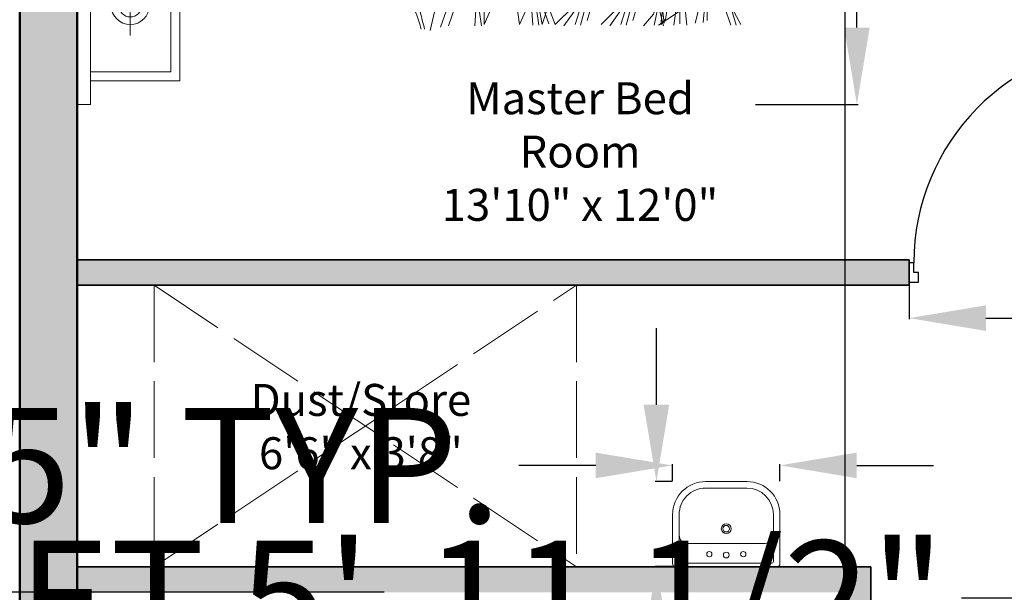
# Model space of a CAD drawing. Units: inches. Extents: x 2796 to 3603, y 978 to 1787.
# Tile 9 of 15: x 3070 to 3224, y 1456 to 1545. Entities that reach past the tile are written whole.
import ezdxf

# ---------------------------------------------------------------- set-up
doc = ezdxf.new("R2010")
doc.units = ezdxf.units.IN
doc.linetypes.add('ACAD_ISO02W100', pattern=[15, 12, -3])
for name, color, linetype, lineweight in [('A-ANNO-DIMS', 7, 'Continuous', 18), ('A-AREA-IDEN', 7, 'Continuous', 18), ('A-DOOR', 6, 'Continuous', 25), ('A-FLOR-FIXT', 8, 'Continuous', 18), ('A-FLOR-OVHD', 7, 'ACAD_ISO02W100', 18), ('A-WALL-EXTR-PATT', 1, 'Continuous', 13), ('A-WALL-INTR-PATT', 5, 'Continuous', 13), ('Furniture', 2, 'Continuous', 18), ('Inner Wall', 5, 'Continuous', 35), ('Outer Wall', 1, 'Continuous', 50)]:
    doc.layers.add(name, color=color, linetype=linetype, lineweight=lineweight)
doc.styles.get("Standard").update_dxf_attribs({"font": 'arial.ttf'})
doc.dimstyles.get("Standard").update_dxf_attribs({"dimtxt": 18, "dimasz": 12, "dimexe": 0.18, "dimexo": 0.0625, "dimgap": 0.09, "dimtad": 0, "dimtih": 1, "dimtoh": 1, "dimdec": 0, "dimzin": 0, "dimdsep": 46, "dimlunit": 3, "dimtxsty": 'Standard', "dimcen": 0.09, "dimadec": 0, "dimazin": 0, "dimtfac": 1, "dimtdec": 0, "dimtofl": 0, "dimtmove": 0, "dimatfit": 3, "dimfxl": 1, "dimtolj": 1, "dimtzin": 0, "dimarcsym": 0})

# ---------------------------------------------------------------- blocks, each defined once
blk = doc.blocks.new('A$C57EA129C')
for p, q in [((0, 0.4428), (0, 0.1782)), ((0.016, 0.4589), (0.5631, 0.4589)), ((0.0356, 0.4321), (0.0356, 0.2896)), ((0.0445, 0.441), (0.5346, 0.441)), ((0.5435, 0.4321), (0.5435, 0.2896)), ((0.5791, 0.4428), (0.5791, 0.1782)), ((0.0802, 0.3341), (0.499, 0.3341)), ((0.0356, 0.2896), (0.0356, 0.1782)), ((0.5435, 0.2896), (0.5435, 0.1782)), ((0.1782, 0.0356), (0.4009, 0.0356)), ((0.1782, 0), (0.4009, 0))]:
    blk.add_line(p, q)
for centre, radius in [((0.1982, 0.392), 0.0143), ((0.2896, 0.3965), 0.0156), ((0.3809, 0.392), 0.0143), ((0.2896, 0.2545), 0.0267), ((0.2896, 0.2545), 0.0178)]:
    blk.add_circle(centre, radius)
for centre, radius, start, end in [((0.016, 0.4428), 0.016, 90, 180), ((0.0445, 0.4321), 0.00891, 90, 180), ((0.5346, 0.4321), 0.00891, 0, 90), ((0.5631, 0.4428), 0.016, 0, 90), ((0.0802, 0.2896), 0.0445, 90, 180), ((0.499, 0.2896), 0.0445, 0, 90), ((0.1782, 0.1782), 0.1782, 180, 270), ((0.1782, 0.1782), 0.1426, 180, 270), ((0.4009, 0.1782), 0.1782, 270, 0), ((0.4009, 0.1782), 0.1426, 270, 0)]:
    blk.add_arc(centre, radius, start, end)
blk = doc.blocks.new('A$C2B723114')
for p, q in [((0, 2.9047), (2.8274, 2.9047)), ((0, 2.8487), (0, 2.9047)), ((0.4243, 2.8697), (0.4243, 2.4855)), ((2.4742, 2.8697), (2.4742, 2.4855)), ((2.8274, 2.9047), (2.8274, 2.8487)), ((2.8274, 2.8487), (0, 2.8487)), ((0.1012, 2.4649), (0.1012, 2.849)), ((0.1396, 2.5033), (0.1396, 2.849)), ((0.6794, 0.7051), (0.6794, 2.8509)), ((0.7187, 0.7435), (0.7187, 2.8509)), ((2.1776, 2.8509), (2.1776, 0.7454)), ((2.216, 2.8509), (2.216, 0.707)), ((2.6798, 2.5052), (2.6798, 2.8509)), ((2.7182, 2.4668), (2.7182, 2.8509)), ((0.6087, 2.6776), (0.295, 2.6776)), ((2.6586, 2.6776), (2.2821, 2.6776)), ((1.3789, 2.4999), (1.3598, 2.5761)), ((2.0593, 2.4999), (2.0402, 2.5761)), ((0.6766, 2.5033), (0.1396, 2.5033)), ((1.3858, 2.4723), (1.3789, 2.4999)), ((2.0662, 2.4723), (2.0593, 2.4999)), ((2.2188, 2.5052), (2.6798, 2.5052)), ((0.6794, 2.4649), (0.1012, 2.4649)), ((0.7191, 2.47), (2.1778, 2.4719)), ((2.2188, 2.4668), (2.7182, 2.4668)), ((2.1771, 2.3036), (0.718, 2.1685)), ((1.0365, 1.6233), (2.1246, 2.2989)), ((2.2287, 1.6076), (2.2523, 1.5035)), ((0.5047, 1.5819), (0.5353, 1.4945)), ((0.6174, 1.5819), (0.6232, 1.4916)), ((0.6467, 1.5819), (0.6369, 1.5137)), ((0.6571, 1.4945), (0.6571, 1.5765)), ((2.2726, 1.593), (2.3061, 1.5007)), ((2.3067, 1.5881), (2.3373, 1.5007)), ((2.4194, 1.5881), (2.4251, 1.4979)), ((2.4487, 1.5881), (2.4389, 1.5199)), ((2.4591, 1.5007), (2.4591, 1.5828)), ((0.4269, 0.0884), (0.4269, 1.4945)), ((0.4269, 1.4945), (0.6794, 1.4945)), ((2.4685, 1.4964), (2.216, 1.5022)), ((2.4685, 1.4964), (2.4685, 0.0903)), ((0.3172, 1.3923), (0.4213, 1.3687)), ((2.4685, 1.4044), (2.5491, 1.3861)), ((2.4596, 1.3659), (2.552, 1.3324)), ((0.3318, 1.3485), (0.4241, 1.3149)), ((0.3367, 1.3143), (0.4241, 1.2838)), ((2.4645, 1.3318), (2.552, 1.3012)), ((2.4645, 1.2928), (2.5548, 1.2871)), ((2.4645, 1.2635), (2.5328, 1.2733)), ((2.4699, 1.2531), (2.552, 1.2163)), ((2.552, 1.2531), (2.4699, 1.2531)), ((2.5435, 1.2276), (2.4699, 1.2163)), ((0.3367, 1.2016), (0.427, 1.1959)), ((0.3367, 1.1724), (0.405, 1.1821)), ((2.4699, 1.2163), (2.5463, 1.1823)), ((0.4241, 1.162), (0.3421, 1.162)), ((0.3421, 1.162), (0.4241, 1.1252)), ((2.5491, 1.1654), (2.467, 1.1597)), ((2.5463, 1.1455), (2.467, 1.1342)), ((2.5491, 1.1342), (2.4699, 1.1201)), ((2.4699, 1.1201), (2.5491, 1.0946)), ((2.5463, 1.1172), (2.4727, 1.0918)), ((2.5491, 1.0946), (2.4699, 1.0635)), ((2.4699, 1.0635), (2.5491, 0.9842)), ((0.4157, 1.0206), (0.3421, 1.0093)), ((2.4642, 1.0267), (2.552, 0.9644)), ((0.3421, 1.0093), (0.4185, 0.9754)), ((2.4699, 0.9785), (2.552, 0.9531)), ((0.4213, 0.9584), (0.3392, 0.9527)), ((0.4185, 0.9386), (0.3392, 0.9272)), ((2.4642, 0.9389), (2.4869, 0.9276)), ((2.467, 0.9559), (2.552, 0.9333)), ((0.4213, 0.9272), (0.3421, 0.9131)), ((0.3421, 0.9131), (0.4213, 0.8876)), ((0.4213, 0.8876), (0.3421, 0.8565)), ((0.4185, 0.9103), (0.3449, 0.8848)), ((2.4642, 0.8908), (2.5152, 0.8483)), ((2.4869, 0.9276), (2.5265, 0.9163)), ((2.5265, 0.9163), (2.5491, 0.9163)), ((0.3421, 0.8565), (0.4213, 0.7772)), ((2.467, 0.8455), (2.5208, 0.8342)), ((2.5152, 0.8483), (2.5491, 0.837)), ((0.3364, 0.8197), (0.4241, 0.7574)), ((2.4699, 0.8172), (2.4925, 0.7974)), ((2.5491, 0.8087), (2.4699, 0.8172)), ((2.5208, 0.8342), (2.552, 0.8285)), ((2.552, 0.8285), (2.5293, 0.8087)), ((0.3421, 0.7716), (0.4241, 0.7461)), ((2.5491, 0.7606), (2.467, 0.7719)), ((2.4925, 0.7974), (2.535, 0.7889)), ((2.535, 0.7889), (2.552, 0.7861)), ((0.3392, 0.7489), (0.4241, 0.7263)), ((0.359, 0.7206), (0.3987, 0.7093)), ((2.1776, 0.7454), (0.7187, 0.7435)), ((2.4727, 0.7464), (2.467, 0.7408)), ((2.467, 0.7153), (2.5491, 0.7238)), ((2.552, 0.7464), (2.4727, 0.7464)), ((0.3987, 0.7093), (0.4213, 0.7093)), ((2.216, 0.707), (0.6794, 0.7051)), ((0.9938, 0.6115), (1.7555, 0.7064)), ((2.5491, 0.6842), (2.4642, 0.6615)), ((2.552, 0.7096), (2.467, 0.6842)), ((0.3421, 0.6601), (0.4213, 0.5808)), ((2.5491, 0.6672), (2.4755, 0.6587)), ((2.4755, 0.6474), (2.5548, 0.6276)), ((0.3364, 0.6233), (0.4241, 0.561)), ((2.4642, 0.6191), (2.4784, 0.6134)), ((2.467, 0.5993), (2.4869, 0.5964)), ((2.4784, 0.6134), (2.5406, 0.6077)), ((2.4869, 0.5964), (2.552, 0.5964)), ((2.5406, 0.6077), (2.552, 0.6134)), ((0.3392, 0.5525), (0.4241, 0.5299)), ((0.3421, 0.5752), (0.4241, 0.5497)), ((2.467, 0.5313), (2.5491, 0.5596)), ((0.359, 0.5242), (0.3987, 0.5129)), ((2.467, 0.5087), (2.5548, 0.5342)), ((2.5548, 0.5342), (2.4699, 0.4889)), ((0.3364, 0.4785), (0.3874, 0.436)), ((1.4523, 0.5021), (1.1305, 0.4537)), ((0.3392, 0.4332), (0.393, 0.4219)), ((0.3874, 0.436), (0.4213, 0.4247)), ((1.1305, 0.4537), (0.9938, 0.448)), ((0.4213, 0.415), (0.3364, 0.3923)), ((0.4241, 0.2868), (0.3392, 0.415)), ((0.3421, 0.4049), (0.3647, 0.3851)), ((0.4213, 0.3964), (0.3421, 0.4049)), ((0.4213, 0.398), (0.3477, 0.3895)), ((0.3647, 0.3851), (0.4072, 0.3766)), ((0.393, 0.4219), (0.4241, 0.4162)), ((0.4241, 0.4162), (0.4015, 0.3964)), ((2.467, 0.4133), (2.552, 0.4019)), ((2.467, 0.2879), (2.552, 0.4076)), ((0.4213, 0.3377), (0.3392, 0.3491)), ((0.4072, 0.3766), (0.4241, 0.3738)), ((0.3392, 0.2925), (0.4213, 0.3009)), ((0.4241, 0.3236), (0.3449, 0.3236)), ((2.4642, 0.3049), (2.5491, 0.2851)), ((2.467, 0.319), (2.5548, 0.3134)), ((0.3477, 0.2571), (0.427, 0.2373)), ((2.501, 0.2491), (2.5491, 0.2547)), ((0.3506, 0.2231), (0.4128, 0.2175)), ((0.4128, 0.2175), (0.4241, 0.2231)), ((2.467, 0.2179), (2.5605, 0.1981)), ((2.4699, 0.2491), (2.501, 0.2491)), ((0.359, 0.2061), (0.4241, 0.2061)), ((2.467, 0.1981), (2.5491, 0.1613)), ((2.467, 0.184), (2.4982, 0.1755)), ((2.4982, 0.1755), (2.5463, 0.1359)), ((0.3392, 0.1042), (0.4213, 0.1325)), ((2.4699, 0.1302), (2.535, 0.1104)), ((0.3392, 0.0815), (0.427, 0.107)), ((0.427, 0.107), (0.3421, 0.0617)), ((2.4685, 0.0903), (0.4269, 0.0884)), ((0.5106, 0.094), (0.5106, 0.0657)), ((0.5417, 0.094), (0.5474, 0.0572)), ((0.587, 0.0884), (0.604, 0.0346)), ((0.6512, 0.0884), (0.6682, 0.0346)), ((0.713, 0.094), (0.713, 0.0657)), ((0.7334, 0.0943), (0.7503, 0.0434)), ((0.7786, 0.0915), (0.7786, 0.0632)), ((0.8739, 0.0884), (0.8908, 0.0346)), ((0.956, 0.0943), (0.973, 0.0434)), ((1.0013, 0.0915), (1.0013, 0.0632)), ((1.072, 0.0884), (1.089, 0.0346)), ((1.1338, 0.094), (1.1338, 0.0657)), ((1.1542, 0.0943), (1.1712, 0.0434)), ((1.1995, 0.0915), (1.1995, 0.0632)), ((1.4088, 0.094), (1.4088, 0.0657)), ((1.44, 0.094), (1.4456, 0.0572)), ((1.4853, 0.0884), (1.5023, 0.0346)), ((1.5674, 0.0962), (1.5844, 0.0453)), ((1.6127, 0.0934), (1.6127, 0.0651)), ((1.6297, 0.0849), (1.624, 0.0028)), ((1.6721, 0.0877), (1.6693, 0.0623)), ((1.7344, 0.0934), (1.7344, 0.0651)), ((1.7655, 0.0934), (1.7712, 0.0566)), ((1.8108, 0.0877), (1.8278, 0.034)), ((1.8568, 0.0962), (1.8738, 0.0453)), ((1.9342, 0.0962), (1.9512, 0.0453)), ((1.9795, 0.0934), (1.9795, 0.0651)), ((1.9965, 0.0849), (1.9908, 0.0028)), ((2.039, 0.0877), (2.0361, 0.0623)), ((2.1012, 0.0934), (2.1012, 0.0651)), ((2.1324, 0.0934), (2.138, 0.0566)), ((2.1777, 0.0877), (2.1946, 0.034)), ((2.2236, 0.0962), (2.2406, 0.0453)), ((2.2689, 0.0934), (2.2689, 0.0651)), ((2.2859, 0.0849), (2.2802, 0.0028)), ((2.3284, 0.0877), (2.3255, 0.0623)), ((2.3906, 0.0934), (2.3906, 0.0651)), ((2.4218, 0.0934), (2.4274, 0.0566)), ((2.4642, 0.0991), (2.5378, 0.0877)), ((2.467, 0.0877), (2.484, 0.034)), ((2.535, 0.1104), (2.5491, 0.0991)), ((2.5378, 0.0877), (2.5463, 0.0821)), ((0.5106, 0.0657), (0.5077, 0.0063)), ((0.5474, 0.0572), (0.57, 0.0006)), ((0.713, 0.0657), (0.7101, 0.0063)), ((0.7503, 0.0434), (0.773, 0.0037)), ((0.7786, 0.0632), (0.7843, 0.0066)), ((0.973, 0.0434), (0.9957, 0.0037)), ((1.0013, 0.0632), (1.007, 0.0066)), ((1.1338, 0.0657), (1.131, 0.0063)), ((1.1712, 0.0434), (1.1939, 0.0037)), ((1.1995, 0.0632), (1.2052, 0.0066)), ((1.4088, 0.0657), (1.406, 0.0063)), ((1.4456, 0.0572), (1.4683, 0.0006)), ((1.5844, 0.0453), (1.607, 0.0057)), ((1.6127, 0.0651), (1.6184, 0.0085)), ((1.6693, 0.0623), (1.6608, 0.0028)), ((1.7344, 0.0651), (1.7316, 0.0057)), ((1.7712, 0.0566), (1.7938, 0)), ((1.8738, 0.0453), (1.8964, 0.0057)), ((1.9512, 0.0453), (1.9739, 0.0057)), ((1.9795, 0.0651), (1.9852, 0.0085)), ((2.0361, 0.0623), (2.0276, 0.0028)), ((2.1012, 0.0651), (2.0984, 0.0057)), ((2.138, 0.0566), (2.1607, 0)), ((2.2406, 0.0453), (2.2632, 0.0057)), ((2.2689, 0.0651), (2.2746, 0.0085)), ((2.3255, 0.0623), (2.317, 0.0028)), ((2.3906, 0.0651), (2.3878, 0.0057)), ((2.4274, 0.0566), (2.4501, 0)), ((0.604, 0.0346), (0.621, 0.0063)), ((0.6682, 0.0346), (0.6851, 0.0063)), ((0.8908, 0.0346), (0.9078, 0.0063)), ((1.089, 0.0346), (1.106, 0.0063)), ((1.5023, 0.0346), (1.5192, 0.0082)), ((1.8278, 0.034), (1.8448, 0.0057)), ((2.1946, 0.034), (2.2116, 0.0057)), ((2.484, 0.034), (2.501, 0.0057))]:
    blk.add_line(p, q)
for centre, radius in [((0.4243, 2.6776), 0.0821), ((2.4742, 2.6776), 0.0821), ((0.4243, 2.6776), 0.0493), ((2.4742, 2.6776), 0.0493)]:
    blk.add_circle(centre, radius)
for centre, radius, start, end in [((0.8078, 2.821), 0.00214, 160.436, 281.8931), ((0.8088, 2.8207), 0.00315, 111.7883, 160.436), ((0.8162, 2.8021), 0.0232, 94.3025, 111.7883), ((0.8091, 2.8151), 0.00394, 21.9904, 101.8931), ((0.8409, 2.7949), 0.0302, 158.579, 188.1335), ((1.0356, 2.8227), 0.2268, 188.1335, 192.1095), ((0.7994, 2.8112), 0.0144, 338.579, 21.9904), ((0.8165, 2.7987), 0.0266, 59.3487, 94.3025), ((0.8554, 2.8643), 0.0497, 239.3487, 264.7408), ((0.9202, 3.5684), 0.7568, 264.7408, 268.0921), ((0.8679, 2.7254), 0.0915, 74.0648, 94.2159), ((0.8679, 2.7254), 0.0915, 53.9136, 74.0648), ((0.9409, 4.189), 1.3777, 268.0921, 270.5757), ((0.8679, 2.7254), 0.0915, 36.1766, 53.9136), ((0.86, 2.6097), 0.2158, 62.7604, 69.1397), ((0.9466, 3.6164), 0.8051, 270.5757, 274.8018), ((0.9263, 2.7386), 0.0708, 51.6114, 62.7604), ((0.7461, 2.511), 0.3611, 46.1885, 51.6114), ((1.0364, 2.548), 0.2671, 87.4614, 94.8018), ((1.042, 2.6745), 0.1405, 79.8101, 87.4614), ((1.1532, 3.2931), 0.488, 259.8101, 263.9133), ((1.204, 3.7695), 0.9671, 263.9133, 270), ((1.204, 3.4318), 0.6294, 270, 277.5469), ((1.2573, 3.0292), 0.2233, 277.5469, 285.744), ((1.3941, 2.5438), 0.281, 98.4372, 105.744), ((1.3747, 2.6748), 0.1486, 90, 98.4372), ((1.3713, 2.8186), 0.0315, 274.4002, 333.4195), ((0.923, 2.7382), 0.4535, 0, 6.2324), ((1.3747, 2.74), 0.0833, 78.7276, 90), ((1.3886, 2.8099), 0.0121, 333.4195, 78.7276), ((1.4882, 2.821), 0.00214, 160.436, 281.8931), ((1.4892, 2.8207), 0.00315, 111.7883, 160.436), ((1.4966, 2.8021), 0.0232, 94.3025, 111.7883), ((1.4895, 2.8151), 0.00394, 21.9904, 101.8931), ((1.5213, 2.7949), 0.0302, 158.579, 188.1335), ((1.716, 2.8227), 0.2268, 188.1335, 192.1095), ((1.4798, 2.8112), 0.0144, 338.579, 21.9904), ((1.4969, 2.7987), 0.0266, 59.3487, 94.3025), ((1.5358, 2.8643), 0.0497, 239.3487, 264.7408), ((1.6006, 3.5684), 0.7568, 264.7408, 268.0921), ((1.5483, 2.7254), 0.0915, 74.0648, 94.2159), ((1.5483, 2.7254), 0.0915, 53.9136, 74.0648), ((1.6213, 4.189), 1.3777, 268.0921, 270.5757), ((1.5483, 2.7254), 0.0915, 36.1766, 53.9136), ((1.5404, 2.6097), 0.2158, 62.7604, 69.1397), ((1.627, 3.6164), 0.8051, 270.5757, 274.8018), ((1.6067, 2.7386), 0.0708, 51.6114, 62.7604), ((1.4265, 2.511), 0.3611, 46.1885, 51.6114), ((1.7168, 2.548), 0.2671, 87.4614, 94.8018), ((1.7224, 2.6745), 0.1405, 79.8101, 87.4614), ((1.8336, 3.2931), 0.488, 259.8101, 263.9133), ((1.8844, 3.7695), 0.9671, 263.9133, 270), ((1.8844, 3.4318), 0.6294, 270, 277.5469), ((1.9377, 3.0292), 0.2233, 277.5469, 285.744), ((2.0745, 2.5438), 0.281, 98.4372, 105.744), ((2.0551, 2.6748), 0.1486, 90, 98.4372), ((2.0517, 2.8186), 0.0315, 274.4002, 333.4195), ((1.6034, 2.7382), 0.4535, 0, 6.2324), ((2.0551, 2.74), 0.0833, 78.7276, 90), ((2.069, 2.8099), 0.0121, 333.4195, 78.7276), ((0.635, 2.7368), 0.1829, 7.6809, 12.1095), ((-0.0181, 2.6487), 0.8418, 3.3687, 7.6809), ((0.8679, 2.7254), 0.0915, 18.4397, 36.1766), ((0.8523, 2.6218), 0.2076, 39.0349, 46.1885), ((0.9783, 2.7239), 0.0455, 28.3168, 39.0349), ((0.8558, 2.6579), 0.1846, 23.0028, 28.3168), ((1.3154, 2.7368), 0.1829, 7.6809, 12.1095), ((0.6623, 2.6487), 0.8418, 3.3687, 7.6809), ((1.5483, 2.7254), 0.0915, 18.4397, 36.1766), ((1.5327, 2.6218), 0.2076, 39.0349, 46.1885), ((1.6587, 2.7239), 0.0455, 28.3168, 39.0349), ((1.5362, 2.6579), 0.1846, 23.0028, 28.3168), ((0.5722, 2.8434), 0.8132, 347.8016, 350.3156), ((1.1884, 2.7382), 0.1881, 350.3156, 0), ((1.2526, 2.8434), 0.8132, 347.8016, 350.3156), ((1.8688, 2.7382), 0.1881, 350.3156, 0), ((0.1976, 2.6614), 0.6258, 358.3669, 3.3687), ((1.6528, 2.6098), 0.2924, 167.8016, 171.9949), ((0.878, 2.6614), 0.6258, 358.3669, 3.3687), ((2.3332, 2.6098), 0.2924, 167.8016, 171.9949), ((-0.4351, 2.6794), 1.2587, 356.945, 358.3669), ((1.9648, 2.5659), 0.6074, 171.9949, 177.3351), ((0.2453, 2.6794), 1.2587, 356.945, 358.3669), ((2.6452, 2.5659), 0.6074, 171.9949, 177.3351), ((-11.7321, 3.2823), 12.5718, 356.49514, 356.94504), ((1.4204, 2.5912), 0.0624, 177.3351, 194.0452), ((-11.0517, 3.2823), 12.5718, 356.49514, 356.94504), ((2.1008, 2.5912), 0.0624, 177.3351, 194.0452), ((0.5206, 2.5319), 0.2961, 350.0016, 356.4951), ((1.4917, 3.1364), 0.681, 244.6889, 246.5156), ((1.4917, 3.1364), 0.681, 246.5156, 248.3423), ((1.4917, 3.1364), 0.681, 248.3423, 250.572), ((1.4917, 3.1364), 0.681, 250.572, 252.8018), ((1.201, 2.5319), 0.2961, 350.0016, 356.4951), ((2.1721, 3.1364), 0.681, 244.6889, 246.5156), ((2.1721, 3.1364), 0.681, 246.5156, 248.3423), ((2.1721, 3.1364), 0.681, 248.3423, 250.572), ((2.1721, 3.1364), 0.681, 250.572, 252.8018), ((0.8298, 2.4774), 0.0178, 170.0016, 196.6978), ((0.8139, 2.4726), 0.00122, 196.6978, 277.1204), ((0.8041, 2.5514), 0.0807, 277.1204, 286.2212), ((0.8068, 2.5419), 0.0707, 286.2212, 297.2841), ((0.8584, 2.4419), 0.0418, 102.869, 117.2841), ((0.879, 2.3515), 0.1345, 93.574, 102.869), ((0.9376, 1.4146), 1.0732, 90.2865, 93.574), ((0.9586, -2.7845), 5.2724, 89.0296, 90.2865), ((0.9954, -0.6123), 3.0999, 87.3904, 89.0296), ((1.0854, 1.364), 1.1216, 85.3824, 87.3904), ((1.28, 3.7729), 1.2952, 265.3824, 267.2509), ((1.228, 2.691), 0.2121, 267.2509, 281.5586), ((1.2975, 2.3514), 0.1345, 83.5659, 101.5586), ((1.3002, 2.3754), 0.1104, 72.6136, 83.5659), ((1.3965, 2.6828), 0.2118, 252.6136, 260.5159), ((1.4027, 2.7202), 0.2496, 260.5159, 265.9171), ((1.385, 2.4721), 0.000845, 265.9171, 14.0449), ((1.5102, 2.4774), 0.0178, 170.0016, 196.6978), ((1.4943, 2.4726), 0.00122, 196.6978, 277.1204), ((1.4845, 2.5514), 0.0807, 277.1204, 286.2212), ((1.4872, 2.5419), 0.0707, 286.2212, 297.2841), ((1.5388, 2.4419), 0.0418, 102.869, 117.2841), ((1.5594, 2.3515), 0.1345, 93.574, 102.869), ((1.618, 1.4146), 1.0732, 90.2865, 93.574), ((1.639, -2.7845), 5.2724, 89.0296, 90.2865), ((1.6758, -0.6123), 3.0999, 87.3904, 89.0296), ((1.7658, 1.364), 1.1216, 85.3824, 87.3904), ((1.9604, 3.7729), 1.2952, 265.3824, 267.2509), ((1.9084, 2.691), 0.2121, 267.2509, 281.5586), ((1.9779, 2.3514), 0.1345, 83.5659, 101.5586), ((1.9806, 2.3754), 0.1104, 72.6136, 83.5659), ((2.0769, 2.6828), 0.2118, 252.6136, 260.5159), ((2.0831, 2.7202), 0.2496, 260.5159, 265.9171), ((2.0654, 2.4721), 0.000845, 265.9171, 14.0449)]:
    blk.add_arc(centre, radius, start, end)
blk.add_ellipse((0.4962, 1.9132), major_axis=(0.4887, -0.4605), ratio=0.503305, start_param=0.491272, end_param=1.591113)
for points, knots in [([(0.6768, 1.3104), (0.6615, 1.3339), (0.6315, 1.3797), (0.604, 1.4501), (0.5417, 1.4748), (0.5064, 1.4871), (0.4848, 1.4945)], [0, 0, 0, 0, 110.980521, 216.571322, 273.316778, 363.252298, 363.252298, 363.252298, 363.252298]), ([(2.5548, 1.4853), (2.5314, 1.4757), (2.5031, 1.4641), (2.4737, 1.4555), (2.4685, 1.454)], [0, 0, 0, 0, 98.452083, 119.481049, 119.481049, 119.481049, 119.481049]), ([(0.427, 1.4678), (0.4036, 1.4582), (0.3693, 1.4441), (0.3335, 1.4344), (0.3221, 1.4313)], [0, 0, 0, 0, 98.452083, 144.639601, 144.639601, 144.639601, 144.639601]), ([(0.4241, 1.4423), (0.4031, 1.437), (0.3691, 1.4284), (0.3351, 1.4199), (0.3221, 1.4167)], [0, 0, 0, 0, 84.638756, 136.955563, 136.955563, 136.955563, 136.955563]), ([(2.552, 1.4598), (2.5309, 1.4545), (2.5031, 1.4475), (2.4753, 1.4406), (2.4685, 1.4389)], [0, 0, 0, 0, 84.638756, 111.94623, 111.94623, 111.94623, 111.94623]), ([(2.2145, 1.4211), (2.233, 1.4246), (2.2636, 1.4303), (2.2761, 1.3837), (2.3429, 1.3967), (2.3949, 1.3342), (2.4474, 1.3031), (2.4698, 1.2898)], [0, 0, 0, 0, 61.886907, 102.717887, 145.699352, 284.082577, 386.765171, 386.765171, 386.765171, 386.765171]), ([(0.6768, 1.286), (0.6567, 1.2911), (0.6145, 1.3017), (0.5543, 1.3533), (0.4816, 1.349), (0.4362, 1.3493), (0.4233, 1.3493)], [0, 0, 0, 0, 80.250278, 168.388677, 295.908361, 346.663112, 346.663112, 346.663112, 346.663112]), ([(0.4233, 1.3445), (0.4367, 1.3385), (0.464, 1.3264), (0.5129, 1.2848), (0.5456, 1.2161), (0.6131, 1.2349), (0.6142, 1.1913), (0.6642, 1.1806), (0.674, 1.144), (0.6817, 1.1154)], [0, 0, 0, 0, 56.745495, 115.23739, 254.956954, 286.678662, 337.828324, 366.201072, 468.500395, 468.500395, 468.500395, 468.500395]), ([(2.2145, 1.319), (2.2295, 1.319), (2.2678, 1.3192), (2.3288, 1.2705), (2.4143, 1.279), (2.4535, 1.2403), (2.4662, 1.2278)], [0, 0, 0, 0, 57.155505, 146.33427, 287.936209, 355.396728, 355.396728, 355.396728, 355.396728]), ([(2.3573, 1.127), (2.3656, 1.1759), (2.3758, 1.2352), (2.3371, 1.1853), (2.3602, 1.1713), (2.3768, 1.1612)], [0, 0, 0, 0, 107.853607, 130.728419, 189.220329, 189.220329, 189.220329, 189.220329]), ([(2.2182, 1.2059), (2.2419, 1.1958), (2.3116, 1.1659), (2.342, 1.0552), (2.4266, 1.0223), (2.4474, 0.9811), (2.462, 0.9684), (2.4698, 0.9616)], [0, 0, 0, 0, 97.73655, 287.59661, 389.176293, 423.403759, 463.679181, 463.679181, 463.679181, 463.679181]), ([(2.2145, 1.1476), (2.2246, 1.1286), (2.2575, 1.0666), (2.3612, 1.0009), (2.431, 0.9336), (2.4662, 0.8996)], [0, 0, 0, 0, 83.02987, 271.460712, 463.033803, 463.033803, 463.033803, 463.033803]), ([(0.6817, 0.8034), (0.6673, 0.8119), (0.6341, 0.8315), (0.5785, 0.8518), (0.5349, 0.8973), (0.4828, 0.9461), (0.4518, 0.9879), (0.4331, 1.013)], [0, 0, 0, 0, 65.318952, 150.437229, 226.833166, 307.58338, 429.454095, 429.454095, 429.454095, 429.454095]), ([(0.4282, 0.9448), (0.4547, 0.9353), (0.496, 0.9206), (0.5223, 0.8436), (0.5628, 0.7946), (0.6113, 0.7575), (0.6214, 0.7173), (0.6539, 0.7022), (0.672, 0.6897), (0.6768, 0.6864)], [0, 0, 0, 0, 102.299436, 159.044876, 303.717955, 348.579152, 391.138254, 454.581655, 477.456496, 477.456496, 477.456496, 477.456496]), ([(2.2145, 0.823), (2.227, 0.8201), (2.261, 0.8121), (2.261, 0.7401), (2.3352, 0.7659), (2.379, 0.6836), (2.4336, 0.6521), (2.4662, 0.6334)], [0, 0, 0, 0, 46.747668, 127.438174, 179.649794, 280.561838, 429.605131, 429.605131, 429.605131, 429.605131]), ([(0.4282, 0.74), (0.4347, 0.7029), (0.444, 0.6496), (0.5194, 0.6274), (0.555, 0.5807), (0.5975, 0.5243), (0.6789, 0.5415), (0.677, 0.5095), (0.6768, 0.5061)], [0, 0, 0, 0, 130.791737, 187.537266, 286.231946, 353.673191, 460.023761, 472.712403, 472.712403, 472.712403, 472.712403]), ([(2.2218, 0.7246), (2.2595, 0.716), (2.3548, 0.6945), (2.4265, 0.6268), (2.4698, 0.586)], [0, 0, 0, 0, 148.665024, 375.555892, 375.555892, 375.555892, 375.555892]), ([(2.3719, 0.6737), (2.3738, 0.6431), (2.3772, 0.5878), (2.3146, 0.6382), (2.3401, 0.7015), (2.2971, 0.6649), (2.2923, 0.6965), (2.289, 0.7176)], [0, 0, 0, 0, 83.446591, 150.887818, 201.642461, 230.015204, 286.760644, 286.760644, 286.760644, 286.760644]), ([(0.6768, 0.6864), (0.7275, 0.655), (0.8251, 0.5944), (0.9391, 0.606), (0.9938, 0.6115)], [0, 0, 0, 0, 225.995823, 434.686543, 434.686543, 434.686543, 434.686543]), ([(2.2145, 0.5167), (2.1764, 0.5522), (2.1051, 0.6184), (1.9357, 0.5803), (1.9385, 0.6342), (1.9388, 0.6395)], [0, 0, 0, 0, 208.073343, 389.01094, 409.01094, 409.01094, 409.01094, 409.01094]), ([(0.6768, 0.5061), (0.7554, 0.4794), (0.8591, 0.4442), (0.9675, 0.4473), (0.9938, 0.448)], [0, 0, 0, 0, 319.374611, 421.61723, 421.61723, 421.61723, 421.61723]), ([(0.4331, 0.4427), (0.4498, 0.4356), (0.4827, 0.4216), (0.5314, 0.3759), (0.632, 0.3884), (0.6996, 0.3513), (0.7423, 0.3278)], [0, 0, 0, 0, 70.931849, 139.556414, 248.154027, 434.709995, 434.709995, 434.709995, 434.709995]), ([(2.4625, 0.1088), (2.4095, 0.1438), (2.2904, 0.2226), (2.0623, 0.1771), (1.9006, 0.2246), (1.7699, 0.2337), (1.6941, 0.2766), (1.5528, 0.2786), (1.4005, 0.2587), (1.2324, 0.3267), (1.059, 0.2939), (0.9218, 0.426), (0.7359, 0.3204), (0.5586, 0.2391), (0.4502, 0.3116), (0.427, 0.3272)], [0, 0, 0, 0, 239.874704, 538.942419, 850.40885, 893.390315, 1047.998294, 1176.505142, 1437.500972, 1637.333004, 1864.324391, 2089.058767, 2248.736533, 2637.953392, 2744.252142, 2744.252142, 2744.252142, 2744.252142]), ([(1.9771, 0.0962), (1.9286, 0.1117), (1.7864, 0.157), (1.5223, 0.1992), (1.2611, 0.141), (1.0527, 0.2023), (0.8859, 0.1885), (0.76, 0.3042), (0.6211, 0.292), (0.5187, 0.3203), (0.4572, 0.3456), (0.4282, 0.3575)], [0, 0, 0, 0, 198.710624, 582.73994, 1031.873213, 1206.082894, 1423.278209, 1655.952104, 1808.744089, 1945.69963, 2068.229211, 2068.229211, 2068.229211, 2068.229211]), ([(0.8718, 0.2941), (0.8821, 0.3221), (0.9041, 0.3814), (0.9523, 0.2773), (0.8733, 0.2454), (0.8757, 0.2798), (0.8766, 0.2941)], [0, 0, 0, 0, 82.720021, 175.094899, 237.579423, 282.440623, 282.440623, 282.440623, 282.440623]), ([(0.8474, 0.0943), (0.82, 0.1047), (0.757, 0.1287), (0.6201, 0.1029), (0.4623, 0.1837), (0.4372, 0.2936), (0.4282, 0.3331)], [0, 0, 0, 0, 112.422038, 258.341957, 533.791494, 688.286079, 688.286079, 688.286079, 688.286079]), ([(1.2715, 0.221), (1.3344, 0.2172), (1.4529, 0.21), (1.2971, 0.2665), (1.2756, 0.2284), (1.2715, 0.221)], [0, 0, 0, 0, 150.888188, 283.977876, 315.699589, 315.699589, 315.699589, 315.699589])]:
    blk.add_open_spline(points, degree=3, knots=knots)
blk = doc.blocks.new('*D12')
at = {"layer": 'A-ANNO-DIMS', "color": 0, "lineweight": -2, "transparency": 16777216}
for p, q in [((3070.18, 1736.68), (3041.33, 1736.68)), ((3041.51, 1724.68), (3041.51, 1391.96)), ((3041.51, 1040.68), (3041.51, 1373.4)), ((3070.18, 1028.68), (3041.33, 1028.68))]:
    blk.add_line(p, q, dxfattribs=at)
at = {"layer": 'A-ANNO-DIMS', "color": 0, "transparency": 16777216}
for points in [[(3039.51, 1724.68), (3043.51, 1724.68), (3041.51, 1736.68)], [(3039.51, 1040.68), (3043.51, 1040.68), (3041.51, 1028.68)]]:
    blk.add_solid(points, dxfattribs=at)
at = {"layer": 'Defpoints', "color": 0, "transparency": 16777216}
for p in [(3041.51, 1736.68), (3070.25, 1736.68), (3070.25, 1028.68)]:
    blk.add_point(p, dxfattribs=at)
at = {"layer": 'A-ANNO-DIMS', "color": 0, "transparency": 16777216, "insert": (3041.51, 1382.68), "char_height": 18, "attachment_point": 5}
blk.add_mtext("\\A1;59'", dxfattribs=at)
blk = doc.blocks.new('DOOR-SWING-36IN')
for points in [[(-0.01, 34.5), (-0.01, 0), (-0.76, 0), (-0.76, 34.5)], [(-35.26, -3), (-33.76, -3), (-33.76, -1.5), (-34.51, -1.5), (-34.51, 0), (-35.26, 0)], [(0.74, -3), (-0.76, -3), (-0.76, -1.5), (-0.01, -1.5), (-0.01, 0), (0.74, 0)]]:
    blk.add_lwpolyline(points, close=True)
blk.add_arc((0, 0), 34.51, 91.2592, 180)
blk = doc.blocks.new('*D19')
at = {"layer": 'A-ANNO-DIMS', "color": 0, "lineweight": -2, "transparency": 16777216}
for p, q in [((3209.25, 1504.11), (3209.25, 1498.37)), ((3245.25, 1504.11), (3245.25, 1498.37)), ((3221.25, 1498.55), (3233.25, 1498.55)), ((3245.25, 1498.55), (3257.25, 1498.55))]:
    blk.add_line(p, q, dxfattribs=at)
at = {"layer": 'A-ANNO-DIMS', "color": 0, "transparency": 16777216}
for points in [[(3221.25, 1500.55), (3221.25, 1496.55), (3209.25, 1498.55)], [(3233.25, 1500.55), (3233.25, 1496.55), (3245.25, 1498.55)]]:
    blk.add_solid(points, dxfattribs=at)
at = {"layer": 'Defpoints', "color": 0, "transparency": 16777216}
for p in [(3209.25, 1504.18), (3245.25, 1504.18), (3245.25, 1498.55)]:
    blk.add_point(p, dxfattribs=at)
at = {"layer": 'A-ANNO-DIMS', "color": 0, "transparency": 16777216, "insert": (3312.19, 1498.55), "char_height": 18, "attachment_point": 5}
blk.add_mtext('\\A1;3\'-0" TYP.', dxfattribs=at)
blk = doc.blocks.new('*D22')
at = {"layer": 'A-ANNO-DIMS', "color": 0, "lineweight": -2, "transparency": 16777216}
for p, q in [((3160.28, 1475.52), (3148.28, 1475.52)), ((3172.28, 1473.07), (3172.28, 1475.7)), ((3189.07, 1473.07), (3189.07, 1475.7)), ((3201.07, 1475.52), (3213.07, 1475.52))]:
    blk.add_line(p, q, dxfattribs=at)
at = {"layer": 'A-ANNO-DIMS', "color": 0, "transparency": 16777216}
for points in [[(3160.28, 1477.52), (3160.28, 1473.52), (3172.28, 1475.52)], [(3201.07, 1477.52), (3201.07, 1473.52), (3189.07, 1475.52)]]:
    blk.add_solid(points, dxfattribs=at)
at = {"layer": 'Defpoints', "color": 0, "transparency": 16777216}
for p in [(3172.28, 1475.52), (3172.28, 1473), (3189.07, 1473)]:
    blk.add_point(p, dxfattribs=at)
at = {"layer": 'A-ANNO-DIMS', "color": 0, "transparency": 16777216, "insert": (3052.51, 1475.52), "char_height": 18, "attachment_point": 5}
blk.add_mtext('\\A1;BASIN 1\'-5" TYP.', dxfattribs=at)
blk = doc.blocks.new('*D23')
at = {"layer": 'A-ANNO-DIMS', "color": 0, "lineweight": -2, "transparency": 16777216}
for p, q in [((3169.76, 1485), (3169.76, 1497)), ((3172.22, 1473), (3169.58, 1473)), ((3172.22, 1459.7), (3169.58, 1459.7)), ((3169.76, 1447.7), (3169.76, 1435.7)), ((3169.76, 1435.7), (3157.76, 1435.7))]:
    blk.add_line(p, q, dxfattribs=at)
at = {"layer": 'A-ANNO-DIMS', "color": 0, "transparency": 16777216}
for points in [[(3167.76, 1485), (3171.76, 1485), (3169.76, 1473)], [(3167.76, 1447.7), (3171.76, 1447.7), (3169.76, 1459.7)]]:
    blk.add_solid(points, dxfattribs=at)
at = {"layer": 'Defpoints', "color": 0, "transparency": 16777216}
for p in [(3172.28, 1473), (3169.76, 1459.7), (3172.28, 1459.7)]:
    blk.add_point(p, dxfattribs=at)
at = {"layer": 'A-ANNO-DIMS', "color": 0, "transparency": 16777216, "insert": (3082.69, 1435.7), "char_height": 18, "attachment_point": 5}
blk.add_mtext('\\A1;1\'-1 1/2" TYP.', dxfattribs=at)
blk = doc.blocks.new('*D27')
at = {"layer": 'A-ANNO-DIMS', "color": 0, "lineweight": -2, "transparency": 16777216}
for p, q in [((3185.26, 1635.1), (3201.27, 1635.1)), ((3201.09, 1623.1), (3201.09, 1592.81)), ((3201.09, 1543.97), (3201.09, 1574.25)), ((3185.26, 1531.97), (3201.27, 1531.97))]:
    blk.add_line(p, q, dxfattribs=at)
at = {"layer": 'A-ANNO-DIMS', "color": 0, "transparency": 16777216}
for points in [[(3199.09, 1623.1), (3203.09, 1623.1), (3201.09, 1635.1)], [(3199.09, 1543.97), (3203.09, 1543.97), (3201.09, 1531.97)]]:
    blk.add_solid(points, dxfattribs=at)
at = {"layer": 'Defpoints', "color": 0, "transparency": 16777216}
for p in [(3185.2, 1635.1), (3201.09, 1635.1), (3185.2, 1531.97)]:
    blk.add_point(p, dxfattribs=at)
at = {"layer": 'A-ANNO-DIMS', "color": 0, "transparency": 16777216, "insert": (3201.09, 1583.53), "char_height": 18, "attachment_point": 5}
blk.add_mtext('\\A1;8\'-7" TYP.', dxfattribs=at)
blk = doc.blocks.new('*D32')
at = {"layer": 'A-ANNO-DIMS', "color": 0, "lineweight": -2, "transparency": 16777216}
for p, q in [((3229.46, 1454.75), (3217.46, 1454.75)), ((3229.46, 1444.07), (3229.46, 1454.93)), ((3289.09, 1454.75), (3241.46, 1454.75)), ((3301.09, 1444.07), (3301.09, 1454.93))]:
    blk.add_line(p, q, dxfattribs=at)
at = {"layer": 'A-ANNO-DIMS', "color": 0, "transparency": 16777216}
for points in [[(3241.46, 1456.75), (3241.46, 1452.75), (3229.46, 1454.75)], [(3289.09, 1456.75), (3289.09, 1452.75), (3301.09, 1454.75)]]:
    blk.add_solid(points, dxfattribs=at)
at = {"layer": 'Defpoints', "color": 0, "transparency": 16777216}
for p in [(3229.46, 1454.75), (3229.46, 1444.01), (3301.09, 1444.01)]:
    blk.add_point(p, dxfattribs=at)
at = {"layer": 'A-ANNO-DIMS', "color": 0, "transparency": 16777216, "insert": (3090.48, 1454.75), "char_height": 18, "attachment_point": 5}
blk.add_mtext('\\A1;DINING SET 5\'-11 1/2"', dxfattribs=at)
blk = doc.blocks.new('*D40')
at = {"layer": 'A-ANNO-DIMS', "color": 0, "lineweight": -2, "transparency": 16777216}
for p, q in [((3079.25, 1455.74), (3079.25, 1775.56)), ((3091.25, 1775.38), (3109.09, 1775.38)), ((3187.25, 1775.38), (3169.41, 1775.38)), ((3199.25, 1455.74), (3199.25, 1775.56))]:
    blk.add_line(p, q, dxfattribs=at)
at = {"layer": 'A-ANNO-DIMS', "color": 0, "transparency": 16777216}
for points in [[(3091.25, 1777.38), (3091.25, 1773.38), (3079.25, 1775.38)], [(3187.25, 1777.38), (3187.25, 1773.38), (3199.25, 1775.38)]]:
    blk.add_solid(points, dxfattribs=at)
at = {"layer": 'Defpoints', "color": 0, "transparency": 16777216}
for p in [(3199.25, 1775.38), (3079.25, 1455.68), (3199.25, 1455.68)]:
    blk.add_point(p, dxfattribs=at)
at = {"layer": 'A-ANNO-DIMS', "color": 0, "transparency": 16777216, "insert": (3139.25, 1775.38), "char_height": 18, "attachment_point": 5}
blk.add_mtext('\\A1;10\'-0"', dxfattribs=at)
blk = doc.blocks.new('*D41')
at = {"layer": 'A-ANNO-DIMS', "color": 0, "lineweight": -2, "transparency": 16777216}
for p, q in [((3079.18, 1455.68), (3031.37, 1455.68)), ((3031.55, 1443.68), (3031.55, 1392.96)), ((3031.55, 1323.68), (3031.55, 1374.4)), ((3079.18, 1311.68), (3031.37, 1311.68))]:
    blk.add_line(p, q, dxfattribs=at)
at = {"layer": 'A-ANNO-DIMS', "color": 0, "transparency": 16777216}
for points in [[(3029.55, 1443.68), (3033.55, 1443.68), (3031.55, 1455.68)], [(3029.55, 1323.68), (3033.55, 1323.68), (3031.55, 1311.68)]]:
    blk.add_solid(points, dxfattribs=at)
at = {"layer": 'Defpoints', "color": 0, "transparency": 16777216}
for p in [(3031.55, 1455.68), (3079.25, 1455.68), (3079.25, 1311.68)]:
    blk.add_point(p, dxfattribs=at)
at = {"layer": 'A-ANNO-DIMS', "color": 0, "transparency": 16777216, "insert": (3031.55, 1383.68), "char_height": 18, "attachment_point": 5}
blk.add_mtext('\\A1;12\'-0"', dxfattribs=at)
blk = doc.blocks.new('*D52')
at = {"layer": 'A-ANNO-DIMS', "color": 0, "lineweight": -2, "transparency": 16777216}
for p, q in [((3031.545499, 1467.67534), (3031.545499, 1479.67534)), ((3127.182999, 1455.67534), (3031.365499, 1455.67534)), ((3127.182999, 1431.67534), (3031.365499, 1431.67534)), ((3031.545499, 1419.67534), (3031.545499, 1407.67534))]:
    blk.add_line(p, q, dxfattribs=at)
at = {"layer": 'A-ANNO-DIMS', "color": 0, "transparency": 16777216}
for points in [[(3029.545499, 1467.67534), (3033.545499, 1467.67534), (3031.545499, 1455.67534)], [(3029.545499, 1419.67534), (3033.545499, 1419.67534), (3031.545499, 1431.67534)]]:
    blk.add_solid(points, dxfattribs=at)
at = {"layer": 'Defpoints', "color": 0, "transparency": 16777216}
for p in [(3031.545499, 1455.67534), (3127.245499, 1455.67534), (3127.245499, 1431.67534)]:
    blk.add_point(p, dxfattribs=at)
at = {"layer": 'A-ANNO-DIMS', "color": 0, "transparency": 16777216, "insert": (3031.545499, 1443.67534), "char_height": 18, "attachment_point": 5}
blk.add_mtext('\\A1;2\'-0"', dxfattribs=at)

msp = doc.modelspace()

# ---------------------------------------------------------------- hatches: boundary and pattern name
at = {"layer": 'A-WALL-EXTR-PATT'}
h = msp.add_hatch(color=256, dxfattribs=at)
h.dxf.hatch_style = 1
h.paths.add_polyline_path([(3424.25, 1736.68), (3070.25, 1736.68), (3070.25, 1106.68), (3227.25, 1106.68), (3227.25, 1115.68), (3226.75, 1115.68), (3223.75, 1115.68), (3079.25, 1115.68), (3079.25, 1727.68), (3127.25, 1727.68), (3415.25, 1727.68), (3415.25, 1188.68), (3424.25, 1188.68)])
h.paths.add_polyline_path([(3291.25, 1032.68), (3074.25, 1032.68), (3074.25, 1106.68), (3070.25, 1106.68), (3070.25, 1028.68), (3291.25, 1028.68)])
h.paths.add_polyline_path([(3291.25, 1115.68), (3281.25, 1115.68), (3281.25, 1106.68), (3291.25, 1106.68)], flags=17)
h.paths.add_polyline_path([(3301.25, 1037.68), (3291.25, 1037.68), (3291.25, 1028.68), (3301.25, 1028.68)])
h.paths.add_polyline_path([(3424.25, 1037.68), (3414.25, 1037.68), (3414.25, 1028.68), (3424.25, 1028.68)])
h.paths.add_polyline_path([(3424.25, 1188.68), (3420.25, 1188.68), (3420.25, 1037.68), (3424.25, 1037.68)])
at = {"layer": 'A-WALL-INTR-PATT'}
h = msp.add_hatch(color=256, dxfattribs=at)
h.dxf.hatch_style = 1
h.paths.add_polyline_path([(3249.25, 1727.68), (3245.25, 1727.68), (3245.25, 1655.68), (3103.25, 1655.68), (3103.25, 1651.68), (3245.25, 1651.68), (3245.25, 1503.68), (3249.25, 1503.68)])
h.paths.add_polyline_path([(3131.25, 1727.68), (3127.25, 1727.68), (3127.25, 1703.68), (3127.25, 1679.68), (3131.25, 1679.68)], flags=17)
h.paths.add_polyline_path([(3391.25, 1655.68), (3325.25, 1655.68), (3325.25, 1727.68), (3321.25, 1727.68), (3321.25, 1655.68), (3273.25, 1655.68), (3273.25, 1651.68), (3391.25, 1651.68)])
h.paths.add_polyline_path([(3203.25, 1459.68), (3079.25, 1459.68), (3079.25, 1455.68), (3199.25, 1455.68), (3199.25, 1431.68), (3199.25, 1347.68), (3203.25, 1347.68)])
h.paths.add_polyline_path([(3209.25, 1507.68), (3079.25, 1507.68), (3079.25, 1503.68), (3209.25, 1503.68)])
h.paths.add_polyline_path([(3415.25, 1507.68), (3285.25, 1507.68), (3285.25, 1503.68), (3415.25, 1503.68)])
h.paths.add_polyline_path([(3415.25, 1459.68), (3333.25, 1459.68), (3333.25, 1455.68), (3415.25, 1455.68)])
h.paths.add_polyline_path([(3291.25, 1311.68), (3287.25, 1311.68), (3287.25, 1192.68), (3227.25, 1192.68), (3227.25, 1267.68), (3263.25, 1267.68), (3263.25, 1271.68), (3223.25, 1271.68), (3223.25, 1151.68), (3227.25, 1151.68), (3227.25, 1188.68), (3291.25, 1188.68)])
h.paths.add_polyline_path([(3227.25, 1311.68), (3079.25, 1311.68), (3079.25, 1307.68), (3227.25, 1307.68)])

# ---------------------------------------------------------------- linework, layer by layer
at = {"layer": 'A-FLOR-OVHD'}
for p, q in [((3091.25, 1503.68), (3091.25, 1459.68)), ((3091.25, 1459.68), (3157.25, 1503.68)), ((3157.25, 1503.68), (3091.25, 1503.68)), ((3091.25, 1503.68), (3157.25, 1459.68)), ((3157.25, 1503.68), (3157.25, 1459.68)), ((3157.25, 1459.68), (3091.25, 1459.68))]:
    msp.add_line(p, q, dxfattribs=at)
at = {"layer": 'Inner Wall'}
for p, q in [((3079.25, 1507.68), (3209.25, 1507.68)), ((3209.25, 1503.68), (3209.25, 1507.68)), ((3079.25, 1503.68), (3209.25, 1503.68)), ((3079.25, 1459.68), (3203.25, 1459.68)), ((3203.25, 1347.68), (3203.25, 1459.68))]:
    msp.add_line(p, q, dxfattribs=at)
at = {"layer": 'Outer Wall'}
for p, q in [((3070.25, 1028.68), (3070.25, 1736.68)), ((3079.25, 1115.68), (3079.25, 1727.68))]:
    msp.add_line(p, q, dxfattribs=at)

# ---------------------------------------------------------------- block references
at = {"layer": 'A-DOOR'}
msp.add_blockref('DOOR-SWING-36IN', (3244.5, 1507.18), dxfattribs=at)
at = {"layer": 'A-FLOR-FIXT', "xscale": 28.98333223671166, "yscale": 28.98333223671166, "zscale": 28.98333223671166, "rotation": 180}
msp.add_blockref('A$C57EA129C', (3189.07, 1473), dxfattribs=at)
at = {"layer": 'Furniture', "xscale": 36.47664764473289, "yscale": 36.47664764473289, "zscale": 36.47664764473289, "rotation": 89.99999999999999}
msp.add_blockref('A$C2B723114', (3185.2, 1531.97), dxfattribs=at)

# ---------------------------------------------------------------- texts
at = {"layer": 'A-AREA-IDEN', "char_height": 5, "attachment_point": 3}
for s, insert in [('\\pxqc;{\\fTimes New Roman|b0|i0|c0|p18;Master Bed Room\\P13\'10" x 12\'0"}', (3185.57, 1535.43)), ('\\pxqc;{\\fTimes New Roman|b0|i0|c0|p18;Dust/Store\\P6\'6" x 3\'8"}', (3151.32, 1488.26))]:
    msp.add_mtext_dynamic_manual_height_columns(s, width=55.5021, gutter_width=12.5, heights=[0], dxfattribs=dict(at, insert=insert))

# ---------------------------------------------------------------- dimensions: what is measured, and where the dimension line sits
at = {"layer": 'A-ANNO-DIMS'}
dim = msp.add_linear_dim(base=(3199.25, 1775.38), p1=(3079.25, 1455.68), p2=(3199.25, 1455.68), dimstyle='Standard', override={"dimdec": 1, "dimlfac": 1, "dimrnd": 0, "dimzin": 1, "dimdsep": 46, "dimlunit": 4, "dimfrac": 2}, dxfattribs=at)
dim.commit()
dim.dimension.update_dxf_attribs({"geometry": '*D40', "text_midpoint": (3139.25, 1775.38)})
for base, p1, p2, override, picture, middle in [((3041.51, 1736.68), (3070.25, 1028.68), (3070.25, 1736.68), {"dimclrd": 0, "dimclre": 0, "dimclrt": 0}, '*D12', (3041.51, 1382.68)), ((3031.55, 1455.68), (3127.25, 1431.68), (3127.25, 1455.68), {"dimdec": 1, "dimlfac": 1, "dimrnd": 0, "dimzin": 1, "dimdsep": 46, "dimlunit": 4, "dimfrac": 2}, '*D52', (3031.55, 1443.68)), ((3031.55, 1455.68), (3079.25, 1311.68), (3079.25, 1455.68), {"dimdec": 1, "dimlfac": 1, "dimrnd": 0, "dimzin": 1, "dimdsep": 46, "dimlunit": 4, "dimfrac": 2}, '*D41', (3031.55, 1383.68))]:
    dim = msp.add_linear_dim(base=base, p1=p1, p2=p2, angle=90, dimstyle='Standard', override=override, dxfattribs=at)
    dim.commit()
    dim.dimension.update_dxf_attribs({"geometry": picture, "text_midpoint": middle})
for base, p1, p2, angle, text, picture, middle in [((3201.09, 1635.1), (3185.2, 1531.97), (3185.2, 1635.1), 90, '<> TYP.', '*D27', (3201.09, 1583.53)), ((3172.28, 1475.52), (3189.07, 1473), (3172.28, 1473), 180, 'BASIN <> TYP.', '*D22', (3052.51, 1475.52)), ((3229.46, 1454.75), (3301.09, 1444.01), (3229.46, 1444.01), 180, 'DINING SET <>', '*D32', (3090.48, 1454.75)), ((3169.76, 1459.7), (3172.28, 1473), (3172.28, 1459.7), 270, '<> TYP.', '*D23', (3082.69, 1435.7))]:
    dim = msp.add_linear_dim(base=base, p1=p1, p2=p2, angle=angle, text=text, dimstyle='Standard', override={"dimdec": 1, "dimlfac": 1, "dimrnd": 0, "dimzin": 1, "dimdsep": 46, "dimlunit": 4, "dimfrac": 2}, dxfattribs=at)
    dim.commit()
    dim.dimension.update_dxf_attribs({"geometry": picture, "text_midpoint": middle})
dim = msp.add_linear_dim(base=(3245.25, 1498.55), p1=(3209.25, 1504.18), p2=(3245.25, 1504.18), text='<> TYP.', dimstyle='Standard', override={"dimdec": 1, "dimlfac": 1, "dimrnd": 0, "dimzin": 1, "dimdsep": 46, "dimlunit": 4, "dimfrac": 2}, dxfattribs=at)
dim.commit()
dim.dimension.update_dxf_attribs({"geometry": '*D19', "text_midpoint": (3312.19, 1498.55)})

doc.saveas('drawing.dxf')
